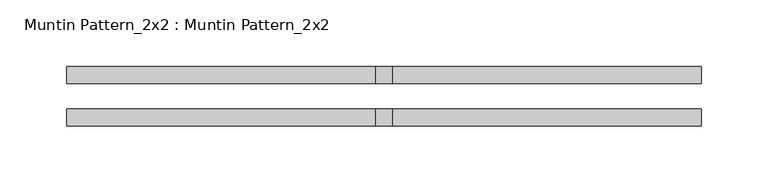
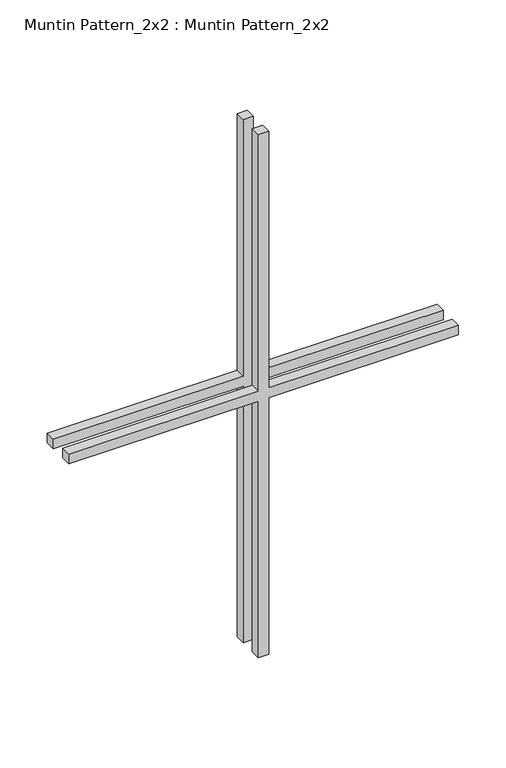
"""IFC4 building model written with IfcOpenShell, lengths in millimetres: proxy geometry, Muntin Pattern_2x2 : Muntin Pattern_2x2."""

from ifc_helpers import new_model, si_unit, frame, origin, place, context, project, spatial, polyline, outline, extrude, source, transform, mapped, element, save


def muntin_pattern_2x2_muntin_pattern_2x2_a56fcb99(model_context):
    return source(origin(), model_context, "Body", "SweptSolid", [
        extrude(outline(polyline([(342.9, -6.35), (342.9, -237.0666667), (330.2, -237.0666667), (330.2, -6.35), (0.0, -6.35), (0.0, 6.35), (330.2, 6.35), (330.2, 237.0666667), (342.9, 237.0666667), (342.9, 6.35), (673.1, 6.35), (673.1, -6.35), (342.9, -6.35)])), frame((0.0, 9.525, 0.0), z_axis=(0.0, 1.0, 0.0), x_axis=(0.0, 0.0, 1.0)), (0.0, 0.0, 1.0), 12.7),
        extrude(outline(polyline([(342.9, -6.35), (342.9, -237.0666667), (330.2, -237.0666667), (330.2, -6.35), (0.0, -6.35), (0.0, 6.35), (330.2, 6.35), (330.2, 237.0666667), (342.9, 237.0666667), (342.9, 6.35), (673.1, 6.35), (673.1, -6.35), (342.9, -6.35)])), frame((0.0, -22.225, 0.0), z_axis=(0.0, 1.0, 0.0), x_axis=(0.0, 0.0, 1.0)), (0.0, 0.0, 1.0), 12.7),
    ])


if __name__ == "__main__":
    model = new_model("IFC4")
    model_context = context("Model", 3, world=origin())
    ifc_project = project(units=[si_unit("LENGTHUNIT", "METRE", prefix="MILLI")], contexts=[model_context])
    site = spatial("IfcSite", under=ifc_project)
    building = spatial("IfcBuilding", under=site)
    placement = place(None, origin())
    muntin_pattern_2x2_muntin_pattern_2x2_shape = muntin_pattern_2x2_muntin_pattern_2x2_a56fcb99(model_context)
    element("IfcBuildingElementProxy", 1, Name="Muntin Pattern_2x2 : Muntin Pattern_2x2", ObjectType="Muntin Pattern_2x2 : Muntin Pattern_2x2", at=placement, inside=building, context=model_context, shape_type="MappedRepresentation", body=[
        mapped(muntin_pattern_2x2_muntin_pattern_2x2_shape, transform((0.0, 0.0, 0.0), x_axis=(1.0, 0.0, 0.0), y_axis=(0.0, 1.0, 0.0), z_axis=(0.0, 0.0, 1.0))),
    ])
    save(model, "model.ifc")

# Revit data of these elements
# Type "Muntin Pattern_2x2 : Muntin Pattern_2x2"
#   Width [instance default] = 4 ft
#   Thickness = 0.041667 ft
#   Height [instance default] = 4 ft
#   Distance = 0.0625 ft
#   Interior Material [instance default] = none
#   Exterior Material [instance default] = none
#   Default Elevation = 0
# Element 1 (IfcBuildingElementProxy, "Muntin Pattern_2x2 : Muntin Pattern_2x2")
#   Width = 1.555556 ft
#   Height = 2.208333 ft
#   Interior Material = Wood - Stained
#   Exterior Material = Clad - White
#   Materials on its faces: "Clad - White", "Wood - Stained"
# Materials
#   "Clad - White": class "Wood", colour RGB 242 242 238, transparency 0, Cost = 0
#   "Wood - Stained": class "Wood", colour RGB 224 178 126, transparency 0, Cost = 0
